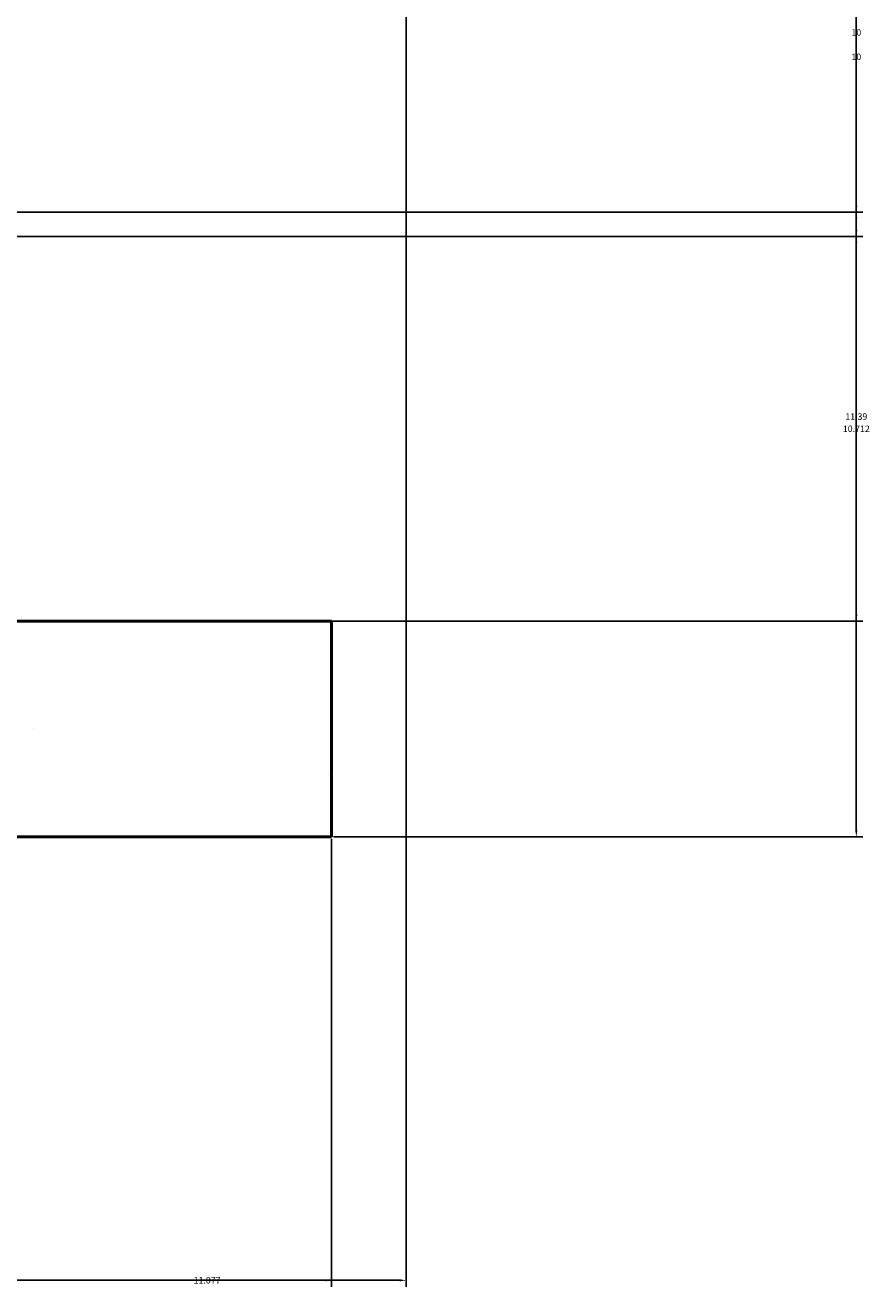
# Model space of a CAD drawing. Units: inches. Extents: x 2812 to 3051, y 1398 to 1659.
# Tile 34 of 65: x 3028 to 3051, y 1398 to 1433. Entities that reach past the tile are written whole.
import ezdxf

# ---------------------------------------------------------------- set-up
doc = ezdxf.new("R2010")
doc.units = ezdxf.units.IN
for name, color, linetype, lineweight in [('A-ANNO-DIMS', 2, 'Continuous', 18), ('S-CONC', 7, 'Continuous', 50), ('S-CONC-PATT', 8, 'Continuous', 18)]:
    doc.layers.add(name, color=color, linetype=linetype, lineweight=lineweight)
doc.styles.get("Standard").update_dxf_attribs({"font": 'arial.ttf'})
doc.dimstyles.get("Standard").update_dxf_attribs({"dimtxt": 0.18, "dimasz": 0.18, "dimexe": 0.18, "dimexo": 0.0625, "dimgap": 0.09, "dimtad": 0, "dimtih": 1, "dimtoh": 1, "dimdec": 4, "dimzin": 0, "dimdsep": 46, "dimtxsty": 'Standard', "dimcen": 0.09, "dimadec": 0, "dimazin": 0, "dimtfac": 1, "dimtdec": 4, "dimtofl": 0, "dimtmove": 0, "dimatfit": 3, "dimfxl": 1, "dimtolj": 1, "dimtzin": 0, "dimarcsym": 0})

# ---------------------------------------------------------------- blocks, each defined once
blk = doc.blocks.new('*D34')
at = {"layer": 'A-ANNO-DIMS', "color": 0, "lineweight": -2, "transparency": 16777216}
for p, q in [((3038.462, 1593.482), (3038.462, 1397.505)), ((3027.385, 1550.757), (3027.385, 1397.505)), ((3027.565, 1397.685), (3032.468, 1397.685)), ((3038.282, 1397.685), (3033.379, 1397.685))]:
    blk.add_line(p, q, dxfattribs=at)
at = {"layer": 'A-ANNO-DIMS', "color": 0, "transparency": 16777216}
for points in [[(3027.565, 1397.715), (3027.565, 1397.655), (3027.385, 1397.685)], [(3038.282, 1397.715), (3038.282, 1397.655), (3038.462, 1397.685)]]:
    blk.add_solid(points, dxfattribs=at)
at = {"layer": 'Defpoints', "color": 0, "transparency": 16777216}
for p in [(3038.462, 1593.544), (3027.385, 1550.82), (3038.462, 1397.685)]:
    blk.add_point(p, dxfattribs=at)
at = {"layer": 'A-ANNO-DIMS', "color": 0, "transparency": 16777216, "insert": (3032.923, 1397.685), "char_height": 0.18, "attachment_point": 5}
blk.add_mtext('\\A1;11.077', dxfattribs=at)
blk = doc.blocks.new('*D48')
at = {"layer": 'A-ANNO-DIMS', "color": 0, "lineweight": -2, "transparency": 16777216}
for p, q in [((3006.385, 1487.973), (3006.385, 1397.505)), ((3036.385, 1409.973), (3036.385, 1397.505)), ((3006.565, 1397.685), (3021.166, 1397.685)), ((3036.205, 1397.685), (3021.603, 1397.685))]:
    blk.add_line(p, q, dxfattribs=at)
at = {"layer": 'A-ANNO-DIMS', "color": 0, "transparency": 16777216}
for points in [[(3006.565, 1397.715), (3006.565, 1397.655), (3006.385, 1397.685)], [(3036.205, 1397.715), (3036.205, 1397.655), (3036.385, 1397.685)]]:
    blk.add_solid(points, dxfattribs=at)
at = {"layer": 'Defpoints', "color": 0, "transparency": 16777216}
for p in [(3006.385, 1488.035), (3036.385, 1410.035), (3036.385, 1397.685)]:
    blk.add_point(p, dxfattribs=at)
at = {"layer": 'A-ANNO-DIMS', "color": 0, "transparency": 16777216, "insert": (3021.385, 1397.685), "char_height": 0.18, "attachment_point": 5}
blk.add_mtext('\\A1;30', dxfattribs=at)
blk = doc.blocks.new('*D54')
at = {"layer": 'A-ANNO-DIMS', "color": 0, "lineweight": -2, "transparency": 16777216}
for p, q in [((3036.447, 1488.035), (3051.178, 1488.035)), ((3050.998, 1487.855), (3050.998, 1449.217)), ((3050.998, 1410.215), (3050.998, 1448.853)), ((3036.447, 1410.035), (3051.178, 1410.035))]:
    blk.add_line(p, q, dxfattribs=at)
at = {"layer": 'A-ANNO-DIMS', "color": 0, "transparency": 16777216}
for points in [[(3050.968, 1487.855), (3051.028, 1487.855), (3050.998, 1488.035)], [(3050.968, 1410.215), (3051.028, 1410.215), (3050.998, 1410.035)]]:
    blk.add_solid(points, dxfattribs=at)
at = {"layer": 'Defpoints', "color": 0, "transparency": 16777216}
for p in [(3036.385, 1488.035), (3050.998, 1488.035), (3036.385, 1410.035)]:
    blk.add_point(p, dxfattribs=at)
at = {"layer": 'A-ANNO-DIMS', "color": 0, "transparency": 16777216, "insert": (3050.998, 1449.035), "char_height": 0.18, "attachment_point": 5}
blk.add_mtext('\\A1;78', dxfattribs=at)
blk = doc.blocks.new('*D64')
at = {"layer": 'A-ANNO-DIMS', "color": 0, "lineweight": -2, "transparency": 16777216}
for p, q in [((2929.438, 1427.426), (3051.178, 1427.426)), ((3050.998, 1427.246), (3050.998, 1421.913)), ((3050.998, 1416.215), (3050.998, 1421.549)), ((2952.447, 1416.035), (3051.178, 1416.035))]:
    blk.add_line(p, q, dxfattribs=at)
at = {"layer": 'A-ANNO-DIMS', "color": 0, "transparency": 16777216}
for points in [[(3050.968, 1427.246), (3051.028, 1427.246), (3050.998, 1427.426)], [(3050.968, 1416.215), (3051.028, 1416.215), (3050.998, 1416.035)]]:
    blk.add_solid(points, dxfattribs=at)
at = {"layer": 'Defpoints', "color": 0, "transparency": 16777216}
for p in [(2929.375, 1427.426), (3050.998, 1427.426), (2952.385, 1416.035)]:
    blk.add_point(p, dxfattribs=at)
at = {"layer": 'A-ANNO-DIMS', "color": 0, "transparency": 16777216, "insert": (3050.998, 1421.731), "char_height": 0.18, "attachment_point": 5}
blk.add_mtext('\\A1;11.39', dxfattribs=at)
blk = doc.blocks.new('*D65')
at = {"layer": 'A-ANNO-DIMS', "color": 0, "lineweight": -2, "transparency": 16777216}
for p, q in [((2920.62, 1437.426), (3051.178, 1437.426)), ((3050.998, 1437.246), (3050.998, 1432.608)), ((3050.998, 1427.606), (3050.998, 1432.245)), ((2929.438, 1427.426), (3051.178, 1427.426))]:
    blk.add_line(p, q, dxfattribs=at)
at = {"layer": 'A-ANNO-DIMS', "color": 0, "transparency": 16777216}
for points in [[(3050.968, 1437.246), (3051.028, 1437.246), (3050.998, 1437.426)], [(3050.968, 1427.606), (3051.028, 1427.606), (3050.998, 1427.426)]]:
    blk.add_solid(points, dxfattribs=at)
at = {"layer": 'Defpoints', "color": 0, "transparency": 16777216}
for p in [(2920.558, 1437.426), (3050.998, 1437.426), (2929.375, 1427.426)]:
    blk.add_point(p, dxfattribs=at)
at = {"layer": 'A-ANNO-DIMS', "color": 0, "transparency": 16777216, "insert": (3050.998, 1432.426), "char_height": 0.18, "attachment_point": 5}
blk.add_mtext('\\A1;10', dxfattribs=at)
blk = doc.blocks.new('*D78')
at = {"layer": 'A-ANNO-DIMS', "color": 0, "lineweight": -2, "transparency": 16777216}
for p, q in [((3012.899, 1426.747), (3051.178, 1426.747)), ((3050.998, 1426.567), (3050.998, 1421.573)), ((3050.998, 1416.215), (3050.998, 1421.209)), ((3018.447, 1416.035), (3051.178, 1416.035))]:
    blk.add_line(p, q, dxfattribs=at)
at = {"layer": 'A-ANNO-DIMS', "color": 0, "transparency": 16777216}
for points in [[(3050.968, 1426.567), (3051.028, 1426.567), (3050.998, 1426.747)], [(3050.968, 1416.215), (3051.028, 1416.215), (3050.998, 1416.035)]]:
    blk.add_solid(points, dxfattribs=at)
at = {"layer": 'Defpoints', "color": 0, "transparency": 16777216}
for p in [(3012.837, 1426.747), (3050.998, 1426.747), (3018.385, 1416.035)]:
    blk.add_point(p, dxfattribs=at)
at = {"layer": 'A-ANNO-DIMS', "color": 0, "transparency": 16777216, "insert": (3050.998, 1421.391), "char_height": 0.18, "attachment_point": 5}
blk.add_mtext('\\A1;10.712', dxfattribs=at)
blk = doc.blocks.new('*D79')
at = {"layer": 'A-ANNO-DIMS', "color": 0, "lineweight": -2, "transparency": 16777216}
for p, q in [((3003.284, 1436.747), (3051.178, 1436.747)), ((3050.998, 1436.567), (3050.998, 1431.929)), ((3050.998, 1426.927), (3050.998, 1431.565)), ((3012.899, 1426.747), (3051.178, 1426.747))]:
    blk.add_line(p, q, dxfattribs=at)
at = {"layer": 'A-ANNO-DIMS', "color": 0, "transparency": 16777216}
for points in [[(3050.968, 1436.567), (3051.028, 1436.567), (3050.998, 1436.747)], [(3050.968, 1426.927), (3051.028, 1426.927), (3050.998, 1426.747)]]:
    blk.add_solid(points, dxfattribs=at)
at = {"layer": 'Defpoints', "color": 0, "transparency": 16777216}
for p in [(3003.221, 1436.747), (3050.998, 1436.747), (3012.837, 1426.747)]:
    blk.add_point(p, dxfattribs=at)
at = {"layer": 'A-ANNO-DIMS', "color": 0, "transparency": 16777216, "insert": (3050.998, 1431.747), "char_height": 0.18, "attachment_point": 5}
blk.add_mtext('\\A1;10', dxfattribs=at)

msp = doc.modelspace()

# ---------------------------------------------------------------- hatches: boundary and pattern name
at = {"layer": 'S-CONC-PATT'}
h = msp.add_hatch(dxfattribs=at)
h.set_pattern_fill('AR-SAND', color=256, scale=0.3)
h.paths.add_polyline_path([(3036.3849, 1416.0354), (3027.3849, 1416.0354), (2826.3849, 1416.0354), (2826.3849, 1410.0354), (2835.3849, 1410.0354), (3036.3849, 1410.0354)])
h.paths.add_polyline_path([(2970.3849, 1488.0354), (2969.3849, 1488.0354), (2941.3849, 1488.0354), (2941.3849, 1482.0354), (2970.3849, 1482.0354)])
h.paths.add_polyline_path([(3036.3849, 1488.0354), (3035.3849, 1488.0354), (3006.3849, 1488.0354), (3006.3849, 1482.0354), (3027.3849, 1482.0354), (3036.3849, 1482.0354)])
h.paths.add_polyline_path([(3034.3849, 1490.0354), (3008.3849, 1490.0354), (3008.3849, 1489.0354), (3034.3849, 1489.0354)])
h.paths.add_polyline_path([(3035.3849, 1489.0354), (3034.3849, 1489.0354), (3007.3849, 1489.0354), (3007.3849, 1488.0354), (3035.3849, 1488.0354)])
h.paths.add_polyline_path([(2968.3849, 1490.0354), (2943.3849, 1490.0354), (2943.3849, 1489.0354), (2968.3849, 1489.0354)])
h.paths.add_polyline_path([(2969.3849, 1489.0354), (2968.3849, 1489.0354), (2942.3849, 1489.0354), (2942.3849, 1488.0354), (2969.3849, 1488.0354)])
h.paths.add_polyline_path([(2896.3849, 1488.0354), (2826.3849, 1488.0354), (2826.3849, 1482.0354), (2896.3849, 1482.0354)])
h.paths.add_polyline_path([(2895.3849, 1489.0354), (2894.3849, 1489.0354), (2827.3849, 1489.0354), (2827.3849, 1488.0354), (2895.3849, 1488.0354)])
h.paths.add_polyline_path([(2894.3849, 1490.0354), (2828.3849, 1490.0354), (2828.3849, 1489.0354), (2894.3849, 1489.0354)])
h = msp.add_hatch(dxfattribs=at)
h.set_pattern_fill('AR-CONC', color=256, scale=0.3)
h.paths.add_polyline_path([(3036.3849, 1416.0354), (3027.3849, 1416.0354), (2826.3849, 1416.0354), (2826.3849, 1410.0354), (2835.3849, 1410.0354), (3036.3849, 1410.0354)])

# ---------------------------------------------------------------- linework, layer by layer
at = {"layer": 'S-CONC'}
for p, q in [((3027.3849, 1416.0354), (3036.3849, 1416.0354)), ((3036.3849, 1416.0354), (3036.3849, 1410.0354)), ((2835.3849, 1410.0354), (3036.3849, 1410.0354))]:
    msp.add_line(p, q, dxfattribs=at)

# ---------------------------------------------------------------- dimensions: what is measured, and where the dimension line sits
at = {"layer": 'A-ANNO-DIMS'}
for base, p1, p2, override, picture, middle in [((3038.4621, 1397.6854), (3027.3849, 1550.82), (3038.4621, 1593.5441), {"dimdec": 3, "dimlfac": 1, "dimrnd": 0, "dimzin": 0, "dimdsep": 46, "dimlunit": 2}, '*D34', (3032.9235, 1397.6854)), ((3036.3849, 1397.6854), (3006.3849, 1488.0354), (3036.3849, 1410.0354), {"dimdec": 0, "dimlfac": 1, "dimrnd": 0, "dimzin": 0, "dimdsep": 46, "dimlunit": 2}, '*D48', (3021.3849, 1397.6854))]:
    dim = msp.add_linear_dim(base=base, p1=p1, p2=p2, dimstyle='Standard', override=override, dxfattribs=at)
    dim.commit()
    dim.dimension.update_dxf_attribs({"geometry": picture, "text_midpoint": middle})
for base, p1, p2, override, picture, middle in [((3050.998, 1488.0354), (3036.3849, 1410.0354), (3036.3849, 1488.0354), {"dimdec": 0, "dimlfac": 1, "dimrnd": 0, "dimzin": 0, "dimdsep": 46, "dimlunit": 2}, '*D54', (3050.998, 1449.0354)), ((3050.998, 1437.4265), (2929.3751, 1427.4265), (2920.5577, 1437.4265), {"dimdec": 0, "dimlfac": 1, "dimrnd": 0, "dimzin": 0, "dimdsep": 46, "dimlunit": 2}, '*D65', (3050.998, 1432.4265)), ((3050.998, 1436.7474), (3012.8368, 1426.7474), (3003.2213, 1436.7474), {"dimdec": 0, "dimlfac": 1, "dimrnd": 0, "dimzin": 0, "dimdsep": 46, "dimlunit": 2}, '*D79', (3050.998, 1431.7474)), ((3050.998, 1427.4265), (2952.3849, 1416.0354), (2929.3751, 1427.4265), {"dimdec": 2, "dimlfac": 1, "dimrnd": 0, "dimzin": 0, "dimdsep": 46, "dimlunit": 2}, '*D64', (3050.998, 1421.7309)), ((3050.998, 1426.7474), (3018.3849, 1416.0354), (3012.8368, 1426.7474), {"dimdec": 3, "dimlfac": 1, "dimrnd": 0, "dimzin": 0, "dimdsep": 46, "dimlunit": 2}, '*D78', (3050.998, 1421.3914))]:
    dim = msp.add_linear_dim(base=base, p1=p1, p2=p2, angle=90, dimstyle='Standard', override=override, dxfattribs=at)
    dim.commit()
    dim.dimension.update_dxf_attribs({"geometry": picture, "text_midpoint": middle})

doc.saveas('drawing.dxf')
